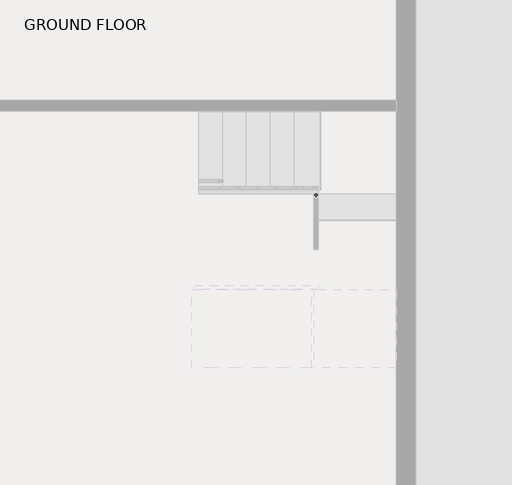
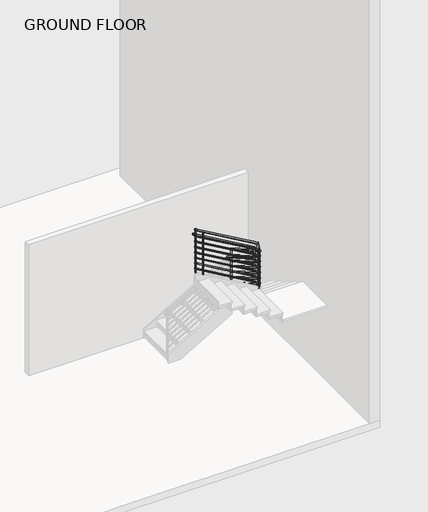
# One storey, part 2 of 3: 1 railing.
"""IFC4 building model written with IfcOpenShell, lengths in millimetres."""

from ifc_helpers import new_model, si_unit, frame, origin, place, context, project, spatial, circle_curve, ellipse_curve, element, save
from ifc_brep_helpers import plane_surface, cylinder_surface, advanced_brep

model = new_model("IFC4")

# Units and contexts
model_context = context("Model", 3, world=origin())
ifc_project = project(units=[si_unit("LENGTHUNIT", "METRE", prefix="MILLI")], contexts=[model_context])

# Site, building, storey
site = spatial("IfcSite", under=ifc_project)
building = spatial("IfcBuilding", under=site)
storey = spatial("IfcBuildingStorey", under=building, Name="GROUND FLOOR", Elevation=304.8)

# Railing
placement = place(None, origin())
element("IfcRailing", 1, ObjectType="Guardrail - Pipe", at=placement, inside=storey, context=model_context, shape_type="AdvancedBrep", body=[
    advanced_brep(
    [(2574.6930349, 4115.4555142, 2326.7540875), (2612.7930349, 4115.4555142, 2326.7540875), (2574.6930349, 3099.4555142, 2913.5348362), (2612.7930349, 3099.4555142, 2913.5348362)],
    [
        (0, 1, ellipse_curve(frame((2593.7430349, 4115.4555142, 2326.7540875), z_axis=(0.0, 1.0, 0.0), x_axis=(0.0, 0.0, -1.0)), 21.9988537, 19.05)),
        (1, 0, ellipse_curve(frame((2593.7430349, 4115.4555142, 2326.7540875), z_axis=(0.0, 1.0, 0.0), x_axis=(0.0, 0.0, -1.0)), 21.9988537, 19.05)),
        (2, 3, ellipse_curve(frame((2593.7430349, 3099.4555142, 2913.5348362), z_axis=(0.0, -0.49993835217939764, 0.8660609932447879), x_axis=(0.0, 0.866060993244788, 0.49993835217939775)), 21.9961413, 19.05)),
        (3, 2, ellipse_curve(frame((2593.7430349, 3099.4555142, 2913.5348362), z_axis=(0.0, -0.49993835217939764, 0.8660609932447879), x_axis=(0.0, 0.866060993244788, 0.49993835217939775)), 21.9961413, 19.05)),
        (0, 2),
        (3, 1),
    ],
    [
        plane_surface(frame((2593.7430349, 4115.4555142, 2348.7529412), z_axis=(0.0, 1.0, 0.0), x_axis=(0.0, 0.0, -1.0))),
        plane_surface(frame((2593.7430349, 3118.5055142, 2924.5315508), z_axis=(0.0, -0.49993835217939764, 0.8660609932447879), x_axis=(1.0, 0.0, 0.0))),
        cylinder_surface(frame((2593.7430349, 4105.9281656, 2332.2565134), z_axis=(0.0, 0.8659542116993035, -0.5001232880402972), x_axis=(1.0, 0.0, 0.0)), 19.05),
    ],
    [
        (0, [[1, 2]]),
        (1, [[3, 4]]),
        (2, [[-1, 5, -4, 6]]),
        (2, [[-2, -6, -3, -5]]),
    ],
),
    advanced_brep(
    [(2574.6930349, 3096.9019419, 2912.0607729), (2612.7930349, 3096.9019419, 2912.0607729), (2574.6930349, 3096.9019419, 3151.9199397), (2612.7930349, 3096.9019419, 3173.913369)],
    [
        (0, 1, ellipse_curve(frame((2593.7430349, 3096.9019419, 2912.0607729), z_axis=(0.0, 0.49993835217939764, -0.8660609932447879), x_axis=(0.0, -0.8660609932447879, -0.49993835217939775)), 21.9961413, 19.05)),
        (1, 0, ellipse_curve(frame((2593.7430349, 3096.9019419, 2912.0607729), z_axis=(0.0, 0.49993835217939764, -0.8660609932447879), x_axis=(0.0, -0.8660609932447879, -0.49993835217939775)), 21.9961413, 19.05)),
        (2, 3, ellipse_curve(frame((2593.7430349, 3096.9019419, 3162.9166543), z_axis=(-0.49993835217939775, 0.0, 0.8660609932447879), x_axis=(-0.8660609932447879, 0.0, -0.49993835217939764)), 21.9961413, 19.05)),
        (3, 2, ellipse_curve(frame((2593.7430349, 3096.9019419, 3162.9166543), z_axis=(-0.49993835217939775, 0.0, 0.8660609932447879), x_axis=(-0.8660609932447879, 0.0, -0.49993835217939764)), 21.9961413, 19.05)),
        (0, 2),
        (3, 1),
    ],
    [
        plane_surface(frame((2593.7430349, 3099.4555142, 2913.5348362), z_axis=(0.0, 0.49993835217939764, -0.8660609932447879), x_axis=(1.0, 0.0, 0.0))),
        plane_surface(frame((2593.7430349, 3099.4555142, 3162.9166543), z_axis=(-0.49993835217939775, 0.0, 0.8660609932447879), x_axis=(0.8660609932447879, 0.0, 0.49993835217939775))),
        cylinder_surface(frame((2593.7430349, 3096.9019419, 2913.5348362), z_axis=(0.0, 0.0, -1.0), x_axis=(1.0, 0.0, 0.0)), 19.05),
    ],
    [
        (0, [[1, 2]]),
        (1, [[3, 4]]),
        (2, [[-1, 5, -4, 6]]),
        (2, [[-2, -6, -3, -5]]),
    ],
),
    advanced_brep(
    [(2593.7430349, 3118.5055142, 3162.9166543), (2593.7430349, 3080.4055142, 3162.9166543), (1247.5430349, 3118.5055142, 3940.4011463), (1247.5430349, 3080.4055142, 3940.4011463)],
    [
        (0, 1, ellipse_curve(frame((2593.7430349, 3099.4555142, 3162.9166543), z_axis=(0.49993835217939775, 0.0, -0.8660609932447879), x_axis=(0.866060993244788, 0.0, 0.49993835217939786)), 21.9961413, 19.05)),
        (1, 0, ellipse_curve(frame((2593.7430349, 3099.4555142, 3162.9166543), z_axis=(0.49993835217939775, 0.0, -0.8660609932447879), x_axis=(0.866060993244788, 0.0, 0.49993835217939786)), 21.9961413, 19.05)),
        (2, 3, ellipse_curve(frame((1247.5430349, 3099.4555142, 3940.4011463), z_axis=(-1.0, 0.0, 0.0), x_axis=(0.0, 0.0, -1.0)), 21.9988537, 19.05)),
        (3, 2, ellipse_curve(frame((1247.5430349, 3099.4555142, 3940.4011463), z_axis=(-1.0, 0.0, 0.0), x_axis=(0.0, 0.0, -1.0)), 21.9988537, 19.05)),
        (0, 2),
        (3, 1),
    ],
    [
        plane_surface(frame((2612.7930349, 3099.4555142, 3173.913369), z_axis=(0.49993835217939775, 0.0, -0.8660609932447879), x_axis=(0.8660609932447879, 0.0, 0.49993835217939775))),
        plane_surface(frame((1247.5430349, 3099.4555142, 3962.4), z_axis=(-1.0, 0.0, 0.0), x_axis=(0.0, -1.0, 0.0))),
        cylinder_surface(frame((2603.2656863, 3099.4555142, 3157.4169413), z_axis=(0.8659542116993035, 0.0, -0.5001232880402972), x_axis=(0.0, -1.0, 0.0)), 19.05),
    ],
    [
        (0, [[1, 2]]),
        (1, [[3, 4]]),
        (2, [[-1, 5, -4, 6]]),
        (2, [[-2, -6, -3, -5]]),
    ],
),
    advanced_brep(
    [(2650.8930349, 4115.4555142, 2479.1540875), (2688.9930349, 4115.4555142, 2479.1540875), (2650.8930349, 3005.9999107, 3119.9091954), (2688.9930349, 3002.5661656, 3121.8923209)],
    [
        (0, 1, ellipse_curve(frame((2669.9430349, 4115.4555142, 2479.1540875), z_axis=(0.0, 1.0, 0.0), x_axis=(0.0, 0.0, -1.0)), 21.9988537, 19.05)),
        (1, 0, ellipse_curve(frame((2669.9430349, 4115.4555142, 2479.1540875), z_axis=(0.0, 1.0, 0.0), x_axis=(0.0, 0.0, -1.0)), 21.9988537, 19.05)),
        (2, 3, ellipse_curve(frame((2669.9430349, 3004.2830381, 3120.9007582), z_axis=(-0.0899527216771524, -0.5009550689581057, 0.8607859935826399), x_axis=(-0.15457437494221507, 0.8608390631720397, 0.4848328267849738)), 22.0408745, 19.05)),
        (3, 2, ellipse_curve(frame((2669.9430349, 3004.2830381, 3120.9007582), z_axis=(-0.0899527216771524, -0.5009550689581057, 0.8607859935826399), x_axis=(-0.15457437494221507, 0.8608390631720397, 0.4848328267849738)), 22.0408745, 19.05)),
        (0, 2),
        (3, 1),
    ],
    [
        plane_surface(frame((2669.9430349, 4115.4555142, 2501.1529412), z_axis=(0.0, 1.0, 0.0), x_axis=(0.0, 0.0, -1.0))),
        plane_surface(frame((2669.9430349, 3023.2555142, 3131.942246), z_axis=(-0.0899527216771524, -0.5009550689581057, 0.8607859935826399), x_axis=(0.995946036621901, -0.04524569628650927, 0.07774521917569083))),
        cylinder_surface(frame((2669.9430349, 4105.9281656, 2484.6565134), z_axis=(0.0, 0.8659542116993035, -0.5001232880402972), x_axis=(1.0, 0.0, 0.0)), 19.05),
    ],
    [
        (0, [[1, 2]]),
        (1, [[3, 4]]),
        (2, [[-1, 5, -4, 6]]),
        (2, [[-2, -6, -3, -5]]),
    ],
),
    advanced_brep(
    [(1247.5430349, 3042.3055142, 4092.8011463), (1247.5430349, 3004.2055142, 4092.8011463), (2649.2536863, 3042.3055142, 3155.5363184), (2652.6874314, 3004.2055142, 3133.7219377), (2627.1390822, 3042.3055142, 3296.0290977), (2627.1390822, 3004.2055142, 3296.0290977)],
    [
        (0, 1, ellipse_curve(frame((1247.5430349, 3023.2555142, 4092.8011463), z_axis=(-1.0, 0.0, 0.0), x_axis=(0.0, 0.0, -1.0)), 21.9988537, 19.05)),
        (1, 0, ellipse_curve(frame((1247.5430349, 3023.2555142, 4092.8011463), z_axis=(-1.0, 0.0, 0.0), x_axis=(0.0, 0.0, -1.0)), 21.9988537, 19.05)),
        (2, 3, ellipse_curve(frame((2650.9705589, 3023.2555142, 3144.6291281), z_axis=(0.0899527216771524, 0.5009550689581057, -0.8607859935826399), x_axis=(0.15457437494221501, -0.8608390631720398, -0.48483282678497347)), 22.0408745, 19.05)),
        (3, 2, ellipse_curve(frame((2650.9705589, 3023.2555142, 3144.6291281), z_axis=(0.0899527216771524, 0.5009550689581057, -0.8607859935826399), x_axis=(0.15457437494221501, -0.8608390631720398, -0.48483282678497347)), 22.0408745, 19.05)),
        (2, 4),
        (4, 5, ellipse_curve(frame((2627.1390822, 3023.2555142, 3296.0290977), z_axis=(0.5659546818459369, 0.0, -0.8244363517559525), x_axis=(-0.824436351755953, 0.0, -0.5659546818459362)), 21.110123, 19.05)),
        (5, 3),
        (5, 4, ellipse_curve(frame((2627.1390822, 3023.2555142, 3296.0290977), z_axis=(0.5659546818459369, 0.0, -0.8244363517559525), x_axis=(-0.824436351755953, 0.0, -0.5659546818459362)), 21.110123, 19.05)),
        (4, 0),
        (1, 5),
    ],
    [
        plane_surface(frame((1247.5430349, 3023.2555142, 4114.8), z_axis=(-1.0, 0.0, 0.0), x_axis=(0.0, -1.0, 0.0))),
        plane_surface(frame((2669.9430349, 3023.2555142, 3146.6117647), z_axis=(0.0899527216771524, 0.5009550689581057, -0.8607859935826399), x_axis=(0.995946036621901, -0.04524569628650927, 0.07774521917569083))),
        cylinder_surface(frame((2651.1247398, 3023.2555142, 3143.6496257), z_axis=(0.1554928635658915, 0.0, -0.9878370155952242), x_axis=(0.0, -1.0, 0.0)), 19.05),
        cylinder_surface(frame((2635.0156863, 3023.2555142, 3291.4800429), z_axis=(0.8659542116993035, 0.0, -0.500123288040297), x_axis=(0.0, -1.0, 0.0)), 19.05),
    ],
    [
        (0, [[1, 2]]),
        (1, [[3, 4]]),
        (2, [[-3, 5, 6, 7]]),
        (2, [[-4, -7, 8, -5]]),
        (3, [[-6, 9, -2, 10]]),
        (3, [[-8, -10, -1, -9]]),
    ],
),
    advanced_brep(
    [(2657.2430349, 4115.4555142, 2334.0870387), (2682.6430349, 4115.4555142, 2334.0870387), (2657.2430349, 3035.9555142, 2957.5415842), (2682.6430349, 3035.9555142, 2957.5415842)],
    [
        (0, 1, ellipse_curve(frame((2669.9430349, 4115.4555142, 2334.0870387), z_axis=(0.0, 1.0, 0.0), x_axis=(0.0, 0.0, -1.0)), 14.6659025, 12.7)),
        (1, 0, ellipse_curve(frame((2669.9430349, 4115.4555142, 2334.0870387), z_axis=(0.0, 1.0, 0.0), x_axis=(0.0, 0.0, -1.0)), 14.6659025, 12.7)),
        (2, 3, ellipse_curve(frame((2669.9430349, 3035.9555142, 2957.5415842), z_axis=(0.0, -1.0, 0.0), x_axis=(0.0, 0.0, -1.0)), 14.6659025, 12.7)),
        (3, 2, ellipse_curve(frame((2669.9430349, 3035.9555142, 2957.5415842), z_axis=(0.0, -1.0, 0.0), x_axis=(0.0, 0.0, -1.0)), 14.6659025, 12.7)),
        (0, 2),
        (3, 1),
    ],
    [
        plane_surface(frame((2669.9430349, 4115.4555142, 2348.7529412), z_axis=(0.0, 1.0, 0.0), x_axis=(0.0, 0.0, -1.0))),
        plane_surface(frame((2669.9430349, 3035.9555142, 2972.2074866), z_axis=(0.0, -1.0, 0.0), x_axis=(0.0, 0.0, -1.0))),
        cylinder_surface(frame((2669.9430349, 4109.1039485, 2337.7553227), z_axis=(0.0, 0.8659542116993035, -0.5001232880402972), x_axis=(1.0, 0.0, 0.0)), 12.7),
    ],
    [
        (0, [[1, 2]]),
        (1, [[3, 4]]),
        (2, [[-1, 5, -4, 6]]),
        (2, [[-2, -6, -3, -5]]),
    ],
),
    advanced_brep(
    [(2682.6430349, 3035.9555142, 2981.5117647), (2682.6430349, 3010.5555142, 2981.5117647), (2659.0857372, 3035.9555142, 2981.5117647), (2659.0857372, 3010.5555142, 2981.5117647), (2644.5430349, 3035.9555142, 3073.9006965), (2644.5430349, 3010.5555142, 3073.9006965)],
    [
        (0, 1, circle_curve(frame((2682.6430349, 3023.2555142, 2981.5117647), z_axis=(1.0, 0.0, 0.0), x_axis=(0.0, -1.0, 0.0)), 12.7)),
        (1, 0, circle_curve(frame((2682.6430349, 3023.2555142, 2981.5117647), z_axis=(1.0, 0.0, 0.0), x_axis=(0.0, -1.0, 0.0)), 12.7)),
        (0, 2),
        (2, 3, ellipse_curve(frame((2659.0857372, 3023.2555142, 2981.5117647), z_axis=(0.7600963305943172, 0.0, -0.6498104094403646), x_axis=(0.6498104094403648, 0.0, 0.7600963305943174)), 16.7084085, 12.7)),
        (3, 1),
        (3, 2, ellipse_curve(frame((2659.0857372, 3023.2555142, 2981.5117647), z_axis=(0.7600963305943172, 0.0, -0.6498104094403646), x_axis=(0.6498104094403648, 0.0, 0.7600963305943174)), 16.7084085, 12.7)),
        (4, 5, ellipse_curve(frame((2644.5430349, 3023.2555142, 3073.9006965), z_axis=(-1.0, 0.0, 0.0), x_axis=(0.0, 0.0, -1.0)), 81.6757741, 12.7)),
        (5, 4, ellipse_curve(frame((2644.5430349, 3023.2555142, 3073.9006965), z_axis=(-1.0, 0.0, 0.0), x_axis=(0.0, 0.0, -1.0)), 81.6757741, 12.7)),
        (2, 4),
        (5, 3),
    ],
    [
        plane_surface(frame((2682.6430349, 3023.2555142, 2994.2117647), z_axis=(1.0, 0.0, 0.0), x_axis=(0.0, -1.0, 0.0))),
        cylinder_surface(frame((2682.6430349, 3023.2555142, 2981.5117647), z_axis=(1.0, 0.0, 0.0), x_axis=(0.0, -1.0, 0.0)), 12.7),
        plane_surface(frame((2644.5430349, 3023.2555142, 3155.5764706), z_axis=(-1.0, 0.0, 0.0), x_axis=(0.0, -1.0, 0.0))),
        cylinder_surface(frame((2657.3975048, 3023.2555142, 2992.2370053), z_axis=(0.15549286356589131, 0.0, -0.9878370155952242), x_axis=(0.0, -1.0, 0.0)), 12.7),
    ],
    [
        (0, [[1, 2]]),
        (1, [[-1, 3, 4, 5]]),
        (1, [[-2, -5, 6, -3]]),
        (2, [[7, 8]]),
        (3, [[-4, 9, -8, 10]]),
        (3, [[-6, -10, -7, -9]]),
    ],
),
    advanced_brep(
    [(2644.5430349, 3035.9555142, 3140.9105681), (2644.5430349, 3010.5555142, 3140.9105681), (1247.5430349, 3035.9555142, 3947.7340975), (1247.5430349, 3010.5555142, 3947.7340975)],
    [
        (0, 1, ellipse_curve(frame((2644.5430349, 3023.2555142, 3140.9105681), z_axis=(1.0, 0.0, 0.0), x_axis=(0.0, 0.0, -1.0)), 14.6659025, 12.7)),
        (1, 0, ellipse_curve(frame((2644.5430349, 3023.2555142, 3140.9105681), z_axis=(1.0, 0.0, 0.0), x_axis=(0.0, 0.0, -1.0)), 14.6659025, 12.7)),
        (2, 3, ellipse_curve(frame((1247.5430349, 3023.2555142, 3947.7340975), z_axis=(-1.0, 0.0, 0.0), x_axis=(0.0, 0.0, -1.0)), 14.6659025, 12.7)),
        (3, 2, ellipse_curve(frame((1247.5430349, 3023.2555142, 3947.7340975), z_axis=(-1.0, 0.0, 0.0), x_axis=(0.0, 0.0, -1.0)), 14.6659025, 12.7)),
        (0, 2),
        (3, 1),
    ],
    [
        plane_surface(frame((2644.5430349, 3023.2555142, 3155.5764706), z_axis=(1.0, 0.0, 0.0), x_axis=(0.0, -1.0, 0.0))),
        plane_surface(frame((1247.5430349, 3023.2555142, 3962.4), z_axis=(-1.0, 0.0, 0.0), x_axis=(0.0, -1.0, 0.0))),
        cylinder_surface(frame((2638.1914692, 3023.2555142, 3144.5788521), z_axis=(0.8659542116993035, 0.0, -0.5001232880402972), x_axis=(0.0, -1.0, 0.0)), 12.7),
    ],
    [
        (0, [[1, 2]]),
        (1, [[3, 4]]),
        (2, [[-1, 5, -4, 6]]),
        (2, [[-2, -6, -3, -5]]),
    ],
),
    advanced_brep(
    [(2657.2430349, 4115.4555142, 2207.0870387), (2682.6430349, 4115.4555142, 2207.0870387), (2657.2430349, 3035.9555142, 2830.5415842), (2682.6430349, 3035.9555142, 2830.5415842)],
    [
        (0, 1, ellipse_curve(frame((2669.9430349, 4115.4555142, 2207.0870387), z_axis=(0.0, 1.0, 0.0), x_axis=(0.0, 0.0, -1.0)), 14.6659025, 12.7)),
        (1, 0, ellipse_curve(frame((2669.9430349, 4115.4555142, 2207.0870387), z_axis=(0.0, 1.0, 0.0), x_axis=(0.0, 0.0, -1.0)), 14.6659025, 12.7)),
        (2, 3, ellipse_curve(frame((2669.9430349, 3035.9555142, 2830.5415842), z_axis=(0.0, -1.0, 0.0), x_axis=(0.0, 0.0, -1.0)), 14.6659025, 12.7)),
        (3, 2, ellipse_curve(frame((2669.9430349, 3035.9555142, 2830.5415842), z_axis=(0.0, -1.0, 0.0), x_axis=(0.0, 0.0, -1.0)), 14.6659025, 12.7)),
        (0, 2),
        (3, 1),
    ],
    [
        plane_surface(frame((2669.9430349, 4115.4555142, 2221.7529412), z_axis=(0.0, 1.0, 0.0), x_axis=(0.0, 0.0, -1.0))),
        plane_surface(frame((2669.9430349, 3035.9555142, 2845.2074866), z_axis=(0.0, -1.0, 0.0), x_axis=(0.0, 0.0, -1.0))),
        cylinder_surface(frame((2669.9430349, 4109.1039485, 2210.7553227), z_axis=(0.0, 0.8659542116993035, -0.5001232880402972), x_axis=(1.0, 0.0, 0.0)), 12.7),
    ],
    [
        (0, [[1, 2]]),
        (1, [[3, 4]]),
        (2, [[-1, 5, -4, 6]]),
        (2, [[-2, -6, -3, -5]]),
    ],
),
    advanced_brep(
    [(2682.6430349, 3035.9555142, 2854.5117647), (2682.6430349, 3010.5555142, 2854.5117647), (2659.0857372, 3035.9555142, 2854.5117647), (2659.0857372, 3010.5555142, 2854.5117647), (2644.5430349, 3035.9555142, 2946.9006965), (2644.5430349, 3010.5555142, 2946.9006965)],
    [
        (0, 1, circle_curve(frame((2682.6430349, 3023.2555142, 2854.5117647), z_axis=(1.0, 0.0, 0.0), x_axis=(0.0, -1.0, 0.0)), 12.7)),
        (1, 0, circle_curve(frame((2682.6430349, 3023.2555142, 2854.5117647), z_axis=(1.0, 0.0, 0.0), x_axis=(0.0, -1.0, 0.0)), 12.7)),
        (0, 2),
        (2, 3, ellipse_curve(frame((2659.0857372, 3023.2555142, 2854.5117647), z_axis=(0.7600963305943172, 0.0, -0.6498104094403646), x_axis=(0.6498104094403648, 0.0, 0.7600963305943174)), 16.7084085, 12.7)),
        (3, 1),
        (3, 2, ellipse_curve(frame((2659.0857372, 3023.2555142, 2854.5117647), z_axis=(0.7600963305943172, 0.0, -0.6498104094403646), x_axis=(0.6498104094403648, 0.0, 0.7600963305943174)), 16.7084085, 12.7)),
        (4, 5, ellipse_curve(frame((2644.5430349, 3023.2555142, 2946.9006965), z_axis=(-1.0, 0.0, 0.0), x_axis=(0.0, 0.0, -1.0)), 81.6757741, 12.7)),
        (5, 4, ellipse_curve(frame((2644.5430349, 3023.2555142, 2946.9006965), z_axis=(-1.0, 0.0, 0.0), x_axis=(0.0, 0.0, -1.0)), 81.6757741, 12.7)),
        (2, 4),
        (5, 3),
    ],
    [
        plane_surface(frame((2682.6430349, 3023.2555142, 2867.2117647), z_axis=(1.0, 0.0, 0.0), x_axis=(0.0, -1.0, 0.0))),
        cylinder_surface(frame((2682.6430349, 3023.2555142, 2854.5117647), z_axis=(1.0, 0.0, 0.0), x_axis=(0.0, -1.0, 0.0)), 12.7),
        plane_surface(frame((2644.5430349, 3023.2555142, 3028.5764706), z_axis=(-1.0, 0.0, 0.0), x_axis=(0.0, -1.0, 0.0))),
        cylinder_surface(frame((2657.3975048, 3023.2555142, 2865.2370053), z_axis=(0.15549286356589131, 0.0, -0.9878370155952242), x_axis=(0.0, -1.0, 0.0)), 12.7),
    ],
    [
        (0, [[1, 2]]),
        (1, [[-1, 3, 4, 5]]),
        (1, [[-2, -5, 6, -3]]),
        (2, [[7, 8]]),
        (3, [[-4, 9, -8, 10]]),
        (3, [[-6, -10, -7, -9]]),
    ],
),
    advanced_brep(
    [(2644.5430349, 3035.9555142, 3013.9105681), (2644.5430349, 3010.5555142, 3013.9105681), (1247.5430349, 3035.9555142, 3820.7340975), (1247.5430349, 3010.5555142, 3820.7340975)],
    [
        (0, 1, ellipse_curve(frame((2644.5430349, 3023.2555142, 3013.9105681), z_axis=(1.0, 0.0, 0.0), x_axis=(0.0, 0.0, -1.0)), 14.6659025, 12.7)),
        (1, 0, ellipse_curve(frame((2644.5430349, 3023.2555142, 3013.9105681), z_axis=(1.0, 0.0, 0.0), x_axis=(0.0, 0.0, -1.0)), 14.6659025, 12.7)),
        (2, 3, ellipse_curve(frame((1247.5430349, 3023.2555142, 3820.7340975), z_axis=(-1.0, 0.0, 0.0), x_axis=(0.0, 0.0, -1.0)), 14.6659025, 12.7)),
        (3, 2, ellipse_curve(frame((1247.5430349, 3023.2555142, 3820.7340975), z_axis=(-1.0, 0.0, 0.0), x_axis=(0.0, 0.0, -1.0)), 14.6659025, 12.7)),
        (0, 2),
        (3, 1),
    ],
    [
        plane_surface(frame((2644.5430349, 3023.2555142, 3028.5764706), z_axis=(1.0, 0.0, 0.0), x_axis=(0.0, -1.0, 0.0))),
        plane_surface(frame((1247.5430349, 3023.2555142, 3835.4), z_axis=(-1.0, 0.0, 0.0), x_axis=(0.0, -1.0, 0.0))),
        cylinder_surface(frame((2638.1914692, 3023.2555142, 3017.5788521), z_axis=(0.8659542116993035, 0.0, -0.5001232880402972), x_axis=(0.0, -1.0, 0.0)), 12.7),
    ],
    [
        (0, [[1, 2]]),
        (1, [[3, 4]]),
        (2, [[-1, 5, -4, 6]]),
        (2, [[-2, -6, -3, -5]]),
    ],
),
    advanced_brep(
    [(2657.2430349, 4115.4555142, 2080.0870387), (2682.6430349, 4115.4555142, 2080.0870387), (2657.2430349, 3035.9555142, 2703.5415842), (2682.6430349, 3035.9555142, 2703.5415842)],
    [
        (0, 1, ellipse_curve(frame((2669.9430349, 4115.4555142, 2080.0870387), z_axis=(0.0, 1.0, 0.0), x_axis=(0.0, 0.0, -1.0)), 14.6659025, 12.7)),
        (1, 0, ellipse_curve(frame((2669.9430349, 4115.4555142, 2080.0870387), z_axis=(0.0, 1.0, 0.0), x_axis=(0.0, 0.0, -1.0)), 14.6659025, 12.7)),
        (2, 3, ellipse_curve(frame((2669.9430349, 3035.9555142, 2703.5415842), z_axis=(0.0, -1.0, 0.0), x_axis=(0.0, 0.0, -1.0)), 14.6659025, 12.7)),
        (3, 2, ellipse_curve(frame((2669.9430349, 3035.9555142, 2703.5415842), z_axis=(0.0, -1.0, 0.0), x_axis=(0.0, 0.0, -1.0)), 14.6659025, 12.7)),
        (0, 2),
        (3, 1),
    ],
    [
        plane_surface(frame((2669.9430349, 4115.4555142, 2094.7529412), z_axis=(0.0, 1.0, 0.0), x_axis=(0.0, 0.0, -1.0))),
        plane_surface(frame((2669.9430349, 3035.9555142, 2718.2074866), z_axis=(0.0, -1.0, 0.0), x_axis=(0.0, 0.0, -1.0))),
        cylinder_surface(frame((2669.9430349, 4109.1039485, 2083.7553227), z_axis=(0.0, 0.8659542116993035, -0.5001232880402972), x_axis=(1.0, 0.0, 0.0)), 12.7),
    ],
    [
        (0, [[1, 2]]),
        (1, [[3, 4]]),
        (2, [[-1, 5, -4, 6]]),
        (2, [[-2, -6, -3, -5]]),
    ],
),
    advanced_brep(
    [(2682.6430349, 3035.9555142, 2727.5117647), (2682.6430349, 3010.5555142, 2727.5117647), (2659.0857372, 3035.9555142, 2727.5117647), (2659.0857372, 3010.5555142, 2727.5117647), (2644.5430349, 3035.9555142, 2819.9006965), (2644.5430349, 3010.5555142, 2819.9006965)],
    [
        (0, 1, circle_curve(frame((2682.6430349, 3023.2555142, 2727.5117647), z_axis=(1.0, 0.0, 0.0), x_axis=(0.0, -1.0, 0.0)), 12.7)),
        (1, 0, circle_curve(frame((2682.6430349, 3023.2555142, 2727.5117647), z_axis=(1.0, 0.0, 0.0), x_axis=(0.0, -1.0, 0.0)), 12.7)),
        (0, 2),
        (2, 3, ellipse_curve(frame((2659.0857372, 3023.2555142, 2727.5117647), z_axis=(0.7600963305943172, 0.0, -0.6498104094403646), x_axis=(0.6498104094403648, 0.0, 0.7600963305943174)), 16.7084085, 12.7)),
        (3, 1),
        (3, 2, ellipse_curve(frame((2659.0857372, 3023.2555142, 2727.5117647), z_axis=(0.7600963305943172, 0.0, -0.6498104094403646), x_axis=(0.6498104094403648, 0.0, 0.7600963305943174)), 16.7084085, 12.7)),
        (4, 5, ellipse_curve(frame((2644.5430349, 3023.2555142, 2819.9006965), z_axis=(-1.0, 0.0, 0.0), x_axis=(0.0, 0.0, -1.0)), 81.6757741, 12.7)),
        (5, 4, ellipse_curve(frame((2644.5430349, 3023.2555142, 2819.9006965), z_axis=(-1.0, 0.0, 0.0), x_axis=(0.0, 0.0, -1.0)), 81.6757741, 12.7)),
        (2, 4),
        (5, 3),
    ],
    [
        plane_surface(frame((2682.6430349, 3023.2555142, 2740.2117647), z_axis=(1.0, 0.0, 0.0), x_axis=(0.0, -1.0, 0.0))),
        cylinder_surface(frame((2682.6430349, 3023.2555142, 2727.5117647), z_axis=(1.0, 0.0, 0.0), x_axis=(0.0, -1.0, 0.0)), 12.7),
        plane_surface(frame((2644.5430349, 3023.2555142, 2901.5764706), z_axis=(-1.0, 0.0, 0.0), x_axis=(0.0, -1.0, 0.0))),
        cylinder_surface(frame((2657.3975048, 3023.2555142, 2738.2370053), z_axis=(0.15549286356589131, 0.0, -0.9878370155952242), x_axis=(0.0, -1.0, 0.0)), 12.7),
    ],
    [
        (0, [[1, 2]]),
        (1, [[-1, 3, 4, 5]]),
        (1, [[-2, -5, 6, -3]]),
        (2, [[7, 8]]),
        (3, [[-4, 9, -8, 10]]),
        (3, [[-6, -10, -7, -9]]),
    ],
),
    advanced_brep(
    [(2644.5430349, 3035.9555142, 2886.9105681), (2644.5430349, 3010.5555142, 2886.9105681), (1247.5430349, 3035.9555142, 3693.7340975), (1247.5430349, 3010.5555142, 3693.7340975)],
    [
        (0, 1, ellipse_curve(frame((2644.5430349, 3023.2555142, 2886.9105681), z_axis=(1.0, 0.0, 0.0), x_axis=(0.0, 0.0, -1.0)), 14.6659025, 12.7)),
        (1, 0, ellipse_curve(frame((2644.5430349, 3023.2555142, 2886.9105681), z_axis=(1.0, 0.0, 0.0), x_axis=(0.0, 0.0, -1.0)), 14.6659025, 12.7)),
        (2, 3, ellipse_curve(frame((1247.5430349, 3023.2555142, 3693.7340975), z_axis=(-1.0, 0.0, 0.0), x_axis=(0.0, 0.0, -1.0)), 14.6659025, 12.7)),
        (3, 2, ellipse_curve(frame((1247.5430349, 3023.2555142, 3693.7340975), z_axis=(-1.0, 0.0, 0.0), x_axis=(0.0, 0.0, -1.0)), 14.6659025, 12.7)),
        (0, 2),
        (3, 1),
    ],
    [
        plane_surface(frame((2644.5430349, 3023.2555142, 2901.5764706), z_axis=(1.0, 0.0, 0.0), x_axis=(0.0, -1.0, 0.0))),
        plane_surface(frame((1247.5430349, 3023.2555142, 3708.4), z_axis=(-1.0, 0.0, 0.0), x_axis=(0.0, -1.0, 0.0))),
        cylinder_surface(frame((2638.1914692, 3023.2555142, 2890.5788521), z_axis=(0.8659542116993035, 0.0, -0.5001232880402972), x_axis=(0.0, -1.0, 0.0)), 12.7),
    ],
    [
        (0, [[1, 2]]),
        (1, [[3, 4]]),
        (2, [[-1, 5, -4, 6]]),
        (2, [[-2, -6, -3, -5]]),
    ],
),
    advanced_brep(
    [(2657.2430349, 4115.4555142, 1953.0870387), (2682.6430349, 4115.4555142, 1953.0870387), (2657.2430349, 3035.9555142, 2576.5415842), (2682.6430349, 3035.9555142, 2576.5415842)],
    [
        (0, 1, ellipse_curve(frame((2669.9430349, 4115.4555142, 1953.0870387), z_axis=(0.0, 1.0, 0.0), x_axis=(0.0, 0.0, -1.0)), 14.6659025, 12.7)),
        (1, 0, ellipse_curve(frame((2669.9430349, 4115.4555142, 1953.0870387), z_axis=(0.0, 1.0, 0.0), x_axis=(0.0, 0.0, -1.0)), 14.6659025, 12.7)),
        (2, 3, ellipse_curve(frame((2669.9430349, 3035.9555142, 2576.5415842), z_axis=(0.0, -1.0, 0.0), x_axis=(0.0, 0.0, -1.0)), 14.6659025, 12.7)),
        (3, 2, ellipse_curve(frame((2669.9430349, 3035.9555142, 2576.5415842), z_axis=(0.0, -1.0, 0.0), x_axis=(0.0, 0.0, -1.0)), 14.6659025, 12.7)),
        (0, 2),
        (3, 1),
    ],
    [
        plane_surface(frame((2669.9430349, 4115.4555142, 1967.7529412), z_axis=(0.0, 1.0, 0.0), x_axis=(0.0, 0.0, -1.0))),
        plane_surface(frame((2669.9430349, 3035.9555142, 2591.2074866), z_axis=(0.0, -1.0, 0.0), x_axis=(0.0, 0.0, -1.0))),
        cylinder_surface(frame((2669.9430349, 4109.1039485, 1956.7553227), z_axis=(0.0, 0.8659542116993035, -0.5001232880402972), x_axis=(1.0, 0.0, 0.0)), 12.7),
    ],
    [
        (0, [[1, 2]]),
        (1, [[3, 4]]),
        (2, [[-1, 5, -4, 6]]),
        (2, [[-2, -6, -3, -5]]),
    ],
),
    advanced_brep(
    [(2682.6430349, 3035.9555142, 2600.5117647), (2682.6430349, 3010.5555142, 2600.5117647), (2659.0857372, 3035.9555142, 2600.5117647), (2659.0857372, 3010.5555142, 2600.5117647), (2644.5430349, 3035.9555142, 2692.9006965), (2644.5430349, 3010.5555142, 2692.9006965)],
    [
        (0, 1, circle_curve(frame((2682.6430349, 3023.2555142, 2600.5117647), z_axis=(1.0, 0.0, 0.0), x_axis=(0.0, -1.0, 0.0)), 12.7)),
        (1, 0, circle_curve(frame((2682.6430349, 3023.2555142, 2600.5117647), z_axis=(1.0, 0.0, 0.0), x_axis=(0.0, -1.0, 0.0)), 12.7)),
        (0, 2),
        (2, 3, ellipse_curve(frame((2659.0857372, 3023.2555142, 2600.5117647), z_axis=(0.7600963305943172, 0.0, -0.6498104094403646), x_axis=(0.6498104094403648, 0.0, 0.7600963305943174)), 16.7084085, 12.7)),
        (3, 1),
        (3, 2, ellipse_curve(frame((2659.0857372, 3023.2555142, 2600.5117647), z_axis=(0.7600963305943172, 0.0, -0.6498104094403646), x_axis=(0.6498104094403648, 0.0, 0.7600963305943174)), 16.7084085, 12.7)),
        (4, 5, ellipse_curve(frame((2644.5430349, 3023.2555142, 2692.9006965), z_axis=(-1.0, 0.0, 0.0), x_axis=(0.0, 0.0, -1.0)), 81.6757741, 12.7)),
        (5, 4, ellipse_curve(frame((2644.5430349, 3023.2555142, 2692.9006965), z_axis=(-1.0, 0.0, 0.0), x_axis=(0.0, 0.0, -1.0)), 81.6757741, 12.7)),
        (2, 4),
        (5, 3),
    ],
    [
        plane_surface(frame((2682.6430349, 3023.2555142, 2613.2117647), z_axis=(1.0, 0.0, 0.0), x_axis=(0.0, -1.0, 0.0))),
        cylinder_surface(frame((2682.6430349, 3023.2555142, 2600.5117647), z_axis=(1.0, 0.0, 0.0), x_axis=(0.0, -1.0, 0.0)), 12.7),
        plane_surface(frame((2644.5430349, 3023.2555142, 2774.5764706), z_axis=(-1.0, 0.0, 0.0), x_axis=(0.0, -1.0, 0.0))),
        cylinder_surface(frame((2657.3975048, 3023.2555142, 2611.2370053), z_axis=(0.15549286356589131, 0.0, -0.9878370155952242), x_axis=(0.0, -1.0, 0.0)), 12.7),
    ],
    [
        (0, [[1, 2]]),
        (1, [[-1, 3, 4, 5]]),
        (1, [[-2, -5, 6, -3]]),
        (2, [[7, 8]]),
        (3, [[-4, 9, -8, 10]]),
        (3, [[-6, -10, -7, -9]]),
    ],
),
    advanced_brep(
    [(2644.5430349, 3035.9555142, 2759.9105681), (2644.5430349, 3010.5555142, 2759.9105681), (1247.5430349, 3035.9555142, 3566.7340975), (1247.5430349, 3010.5555142, 3566.7340975)],
    [
        (0, 1, ellipse_curve(frame((2644.5430349, 3023.2555142, 2759.9105681), z_axis=(1.0, 0.0, 0.0), x_axis=(0.0, 0.0, -1.0)), 14.6659025, 12.7)),
        (1, 0, ellipse_curve(frame((2644.5430349, 3023.2555142, 2759.9105681), z_axis=(1.0, 0.0, 0.0), x_axis=(0.0, 0.0, -1.0)), 14.6659025, 12.7)),
        (2, 3, ellipse_curve(frame((1247.5430349, 3023.2555142, 3566.7340975), z_axis=(-1.0, 0.0, 0.0), x_axis=(0.0, 0.0, -1.0)), 14.6659025, 12.7)),
        (3, 2, ellipse_curve(frame((1247.5430349, 3023.2555142, 3566.7340975), z_axis=(-1.0, 0.0, 0.0), x_axis=(0.0, 0.0, -1.0)), 14.6659025, 12.7)),
        (0, 2),
        (3, 1),
    ],
    [
        plane_surface(frame((2644.5430349, 3023.2555142, 2774.5764706), z_axis=(1.0, 0.0, 0.0), x_axis=(0.0, -1.0, 0.0))),
        plane_surface(frame((1247.5430349, 3023.2555142, 3581.4), z_axis=(-1.0, 0.0, 0.0), x_axis=(0.0, -1.0, 0.0))),
        cylinder_surface(frame((2638.1914692, 3023.2555142, 2763.5788521), z_axis=(0.8659542116993035, 0.0, -0.5001232880402972), x_axis=(0.0, -1.0, 0.0)), 12.7),
    ],
    [
        (0, [[1, 2]]),
        (1, [[3, 4]]),
        (2, [[-1, 5, -4, 6]]),
        (2, [[-2, -6, -3, -5]]),
    ],
),
    advanced_brep(
    [(2657.2430349, 4115.4555142, 1826.0870387), (2682.6430349, 4115.4555142, 1826.0870387), (2657.2430349, 3035.9555142, 2449.5415842), (2682.6430349, 3035.9555142, 2449.5415842)],
    [
        (0, 1, ellipse_curve(frame((2669.9430349, 4115.4555142, 1826.0870387), z_axis=(0.0, 1.0, 0.0), x_axis=(0.0, 0.0, -1.0)), 14.6659025, 12.7)),
        (1, 0, ellipse_curve(frame((2669.9430349, 4115.4555142, 1826.0870387), z_axis=(0.0, 1.0, 0.0), x_axis=(0.0, 0.0, -1.0)), 14.6659025, 12.7)),
        (2, 3, ellipse_curve(frame((2669.9430349, 3035.9555142, 2449.5415842), z_axis=(0.0, -1.0, 0.0), x_axis=(0.0, 0.0, -1.0)), 14.6659025, 12.7)),
        (3, 2, ellipse_curve(frame((2669.9430349, 3035.9555142, 2449.5415842), z_axis=(0.0, -1.0, 0.0), x_axis=(0.0, 0.0, -1.0)), 14.6659025, 12.7)),
        (0, 2),
        (3, 1),
    ],
    [
        plane_surface(frame((2669.9430349, 4115.4555142, 1840.7529412), z_axis=(0.0, 1.0, 0.0), x_axis=(0.0, 0.0, -1.0))),
        plane_surface(frame((2669.9430349, 3035.9555142, 2464.2074866), z_axis=(0.0, -1.0, 0.0), x_axis=(0.0, 0.0, -1.0))),
        cylinder_surface(frame((2669.9430349, 4109.1039485, 1829.7553227), z_axis=(0.0, 0.8659542116993035, -0.5001232880402972), x_axis=(1.0, 0.0, 0.0)), 12.7),
    ],
    [
        (0, [[1, 2]]),
        (1, [[3, 4]]),
        (2, [[-1, 5, -4, 6]]),
        (2, [[-2, -6, -3, -5]]),
    ],
),
    advanced_brep(
    [(2682.6430349, 3035.9555142, 2473.5117647), (2682.6430349, 3010.5555142, 2473.5117647), (2659.0857372, 3035.9555142, 2473.5117647), (2659.0857372, 3010.5555142, 2473.5117647), (2644.5430349, 3035.9555142, 2565.9006965), (2644.5430349, 3010.5555142, 2565.9006965)],
    [
        (0, 1, circle_curve(frame((2682.6430349, 3023.2555142, 2473.5117647), z_axis=(1.0, 0.0, 0.0), x_axis=(0.0, -1.0, 0.0)), 12.7)),
        (1, 0, circle_curve(frame((2682.6430349, 3023.2555142, 2473.5117647), z_axis=(1.0, 0.0, 0.0), x_axis=(0.0, -1.0, 0.0)), 12.7)),
        (0, 2),
        (2, 3, ellipse_curve(frame((2659.0857372, 3023.2555142, 2473.5117647), z_axis=(0.7600963305943172, 0.0, -0.6498104094403646), x_axis=(0.6498104094403648, 0.0, 0.7600963305943174)), 16.7084085, 12.7)),
        (3, 1),
        (3, 2, ellipse_curve(frame((2659.0857372, 3023.2555142, 2473.5117647), z_axis=(0.7600963305943172, 0.0, -0.6498104094403646), x_axis=(0.6498104094403648, 0.0, 0.7600963305943174)), 16.7084085, 12.7)),
        (4, 5, ellipse_curve(frame((2644.5430349, 3023.2555142, 2565.9006965), z_axis=(-1.0, 0.0, 0.0), x_axis=(0.0, 0.0, -1.0)), 81.6757741, 12.7)),
        (5, 4, ellipse_curve(frame((2644.5430349, 3023.2555142, 2565.9006965), z_axis=(-1.0, 0.0, 0.0), x_axis=(0.0, 0.0, -1.0)), 81.6757741, 12.7)),
        (2, 4),
        (5, 3),
    ],
    [
        plane_surface(frame((2682.6430349, 3023.2555142, 2486.2117647), z_axis=(1.0, 0.0, 0.0), x_axis=(0.0, -1.0, 0.0))),
        cylinder_surface(frame((2682.6430349, 3023.2555142, 2473.5117647), z_axis=(1.0, 0.0, 0.0), x_axis=(0.0, -1.0, 0.0)), 12.7),
        plane_surface(frame((2644.5430349, 3023.2555142, 2647.5764706), z_axis=(-1.0, 0.0, 0.0), x_axis=(0.0, -1.0, 0.0))),
        cylinder_surface(frame((2657.3975048, 3023.2555142, 2484.2370053), z_axis=(0.15549286356589131, 0.0, -0.9878370155952242), x_axis=(0.0, -1.0, 0.0)), 12.7),
    ],
    [
        (0, [[1, 2]]),
        (1, [[-1, 3, 4, 5]]),
        (1, [[-2, -5, 6, -3]]),
        (2, [[7, 8]]),
        (3, [[-4, 9, -8, 10]]),
        (3, [[-6, -10, -7, -9]]),
    ],
),
    advanced_brep(
    [(2644.5430349, 3035.9555142, 2632.9105681), (2644.5430349, 3010.5555142, 2632.9105681), (1247.5430349, 3035.9555142, 3439.7340975), (1247.5430349, 3010.5555142, 3439.7340975)],
    [
        (0, 1, ellipse_curve(frame((2644.5430349, 3023.2555142, 2632.9105681), z_axis=(1.0, 0.0, 0.0), x_axis=(0.0, 0.0, -1.0)), 14.6659025, 12.7)),
        (1, 0, ellipse_curve(frame((2644.5430349, 3023.2555142, 2632.9105681), z_axis=(1.0, 0.0, 0.0), x_axis=(0.0, 0.0, -1.0)), 14.6659025, 12.7)),
        (2, 3, ellipse_curve(frame((1247.5430349, 3023.2555142, 3439.7340975), z_axis=(-1.0, 0.0, 0.0), x_axis=(0.0, 0.0, -1.0)), 14.6659025, 12.7)),
        (3, 2, ellipse_curve(frame((1247.5430349, 3023.2555142, 3439.7340975), z_axis=(-1.0, 0.0, 0.0), x_axis=(0.0, 0.0, -1.0)), 14.6659025, 12.7)),
        (0, 2),
        (3, 1),
    ],
    [
        plane_surface(frame((2644.5430349, 3023.2555142, 2647.5764706), z_axis=(1.0, 0.0, 0.0), x_axis=(0.0, -1.0, 0.0))),
        plane_surface(frame((1247.5430349, 3023.2555142, 3454.4), z_axis=(-1.0, 0.0, 0.0), x_axis=(0.0, -1.0, 0.0))),
        cylinder_surface(frame((2638.1914692, 3023.2555142, 2636.5788521), z_axis=(0.8659542116993035, 0.0, -0.5001232880402972), x_axis=(0.0, -1.0, 0.0)), 12.7),
    ],
    [
        (0, [[1, 2]]),
        (1, [[3, 4]]),
        (2, [[-1, 5, -4, 6]]),
        (2, [[-2, -6, -3, -5]]),
    ],
),
    advanced_brep(
    [(2657.2430349, 4115.4555142, 1699.0870387), (2682.6430349, 4115.4555142, 1699.0870387), (2657.2430349, 3035.9555142, 2322.5415842), (2682.6430349, 3035.9555142, 2322.5415842)],
    [
        (0, 1, ellipse_curve(frame((2669.9430349, 4115.4555142, 1699.0870387), z_axis=(0.0, 1.0, 0.0), x_axis=(0.0, 0.0, -1.0)), 14.6659025, 12.7)),
        (1, 0, ellipse_curve(frame((2669.9430349, 4115.4555142, 1699.0870387), z_axis=(0.0, 1.0, 0.0), x_axis=(0.0, 0.0, -1.0)), 14.6659025, 12.7)),
        (2, 3, ellipse_curve(frame((2669.9430349, 3035.9555142, 2322.5415842), z_axis=(0.0, -1.0, 0.0), x_axis=(0.0, 0.0, -1.0)), 14.6659025, 12.7)),
        (3, 2, ellipse_curve(frame((2669.9430349, 3035.9555142, 2322.5415842), z_axis=(0.0, -1.0, 0.0), x_axis=(0.0, 0.0, -1.0)), 14.6659025, 12.7)),
        (0, 2),
        (3, 1),
    ],
    [
        plane_surface(frame((2669.9430349, 4115.4555142, 1713.7529412), z_axis=(0.0, 1.0, 0.0), x_axis=(0.0, 0.0, -1.0))),
        plane_surface(frame((2669.9430349, 3035.9555142, 2337.2074866), z_axis=(0.0, -1.0, 0.0), x_axis=(0.0, 0.0, -1.0))),
        cylinder_surface(frame((2669.9430349, 4109.1039485, 1702.7553227), z_axis=(0.0, 0.8659542116993035, -0.5001232880402972), x_axis=(1.0, 0.0, 0.0)), 12.7),
    ],
    [
        (0, [[1, 2]]),
        (1, [[3, 4]]),
        (2, [[-1, 5, -4, 6]]),
        (2, [[-2, -6, -3, -5]]),
    ],
),
    advanced_brep(
    [(2682.6430349, 3035.9555142, 2346.5117647), (2682.6430349, 3010.5555142, 2346.5117647), (2659.0857372, 3035.9555142, 2346.5117647), (2659.0857372, 3010.5555142, 2346.5117647), (2644.5430349, 3035.9555142, 2438.9006965), (2644.5430349, 3010.5555142, 2438.9006965)],
    [
        (0, 1, circle_curve(frame((2682.6430349, 3023.2555142, 2346.5117647), z_axis=(1.0, 0.0, 0.0), x_axis=(0.0, -1.0, 0.0)), 12.7)),
        (1, 0, circle_curve(frame((2682.6430349, 3023.2555142, 2346.5117647), z_axis=(1.0, 0.0, 0.0), x_axis=(0.0, -1.0, 0.0)), 12.7)),
        (0, 2),
        (2, 3, ellipse_curve(frame((2659.0857372, 3023.2555142, 2346.5117647), z_axis=(0.7600963305943172, 0.0, -0.6498104094403646), x_axis=(0.6498104094403648, 0.0, 0.7600963305943174)), 16.7084085, 12.7)),
        (3, 1),
        (3, 2, ellipse_curve(frame((2659.0857372, 3023.2555142, 2346.5117647), z_axis=(0.7600963305943172, 0.0, -0.6498104094403646), x_axis=(0.6498104094403648, 0.0, 0.7600963305943174)), 16.7084085, 12.7)),
        (4, 5, ellipse_curve(frame((2644.5430349, 3023.2555142, 2438.9006965), z_axis=(-1.0, 0.0, 0.0), x_axis=(0.0, 0.0, -1.0)), 81.6757741, 12.7)),
        (5, 4, ellipse_curve(frame((2644.5430349, 3023.2555142, 2438.9006965), z_axis=(-1.0, 0.0, 0.0), x_axis=(0.0, 0.0, -1.0)), 81.6757741, 12.7)),
        (2, 4),
        (5, 3),
    ],
    [
        plane_surface(frame((2682.6430349, 3023.2555142, 2359.2117647), z_axis=(1.0, 0.0, 0.0), x_axis=(0.0, -1.0, 0.0))),
        cylinder_surface(frame((2682.6430349, 3023.2555142, 2346.5117647), z_axis=(1.0, 0.0, 0.0), x_axis=(0.0, -1.0, 0.0)), 12.7),
        plane_surface(frame((2644.5430349, 3023.2555142, 2520.5764706), z_axis=(-1.0, 0.0, 0.0), x_axis=(0.0, -1.0, 0.0))),
        cylinder_surface(frame((2657.3975048, 3023.2555142, 2357.2370053), z_axis=(0.15549286356589131, 0.0, -0.9878370155952242), x_axis=(0.0, -1.0, 0.0)), 12.7),
    ],
    [
        (0, [[1, 2]]),
        (1, [[-1, 3, 4, 5]]),
        (1, [[-2, -5, 6, -3]]),
        (2, [[7, 8]]),
        (3, [[-4, 9, -8, 10]]),
        (3, [[-6, -10, -7, -9]]),
    ],
),
    advanced_brep(
    [(2644.5430349, 3035.9555142, 2505.9105681), (2644.5430349, 3010.5555142, 2505.9105681), (1247.5430349, 3035.9555142, 3312.7340975), (1247.5430349, 3010.5555142, 3312.7340975)],
    [
        (0, 1, ellipse_curve(frame((2644.5430349, 3023.2555142, 2505.9105681), z_axis=(1.0, 0.0, 0.0), x_axis=(0.0, 0.0, -1.0)), 14.6659025, 12.7)),
        (1, 0, ellipse_curve(frame((2644.5430349, 3023.2555142, 2505.9105681), z_axis=(1.0, 0.0, 0.0), x_axis=(0.0, 0.0, -1.0)), 14.6659025, 12.7)),
        (2, 3, ellipse_curve(frame((1247.5430349, 3023.2555142, 3312.7340975), z_axis=(-1.0, 0.0, 0.0), x_axis=(0.0, 0.0, -1.0)), 14.6659025, 12.7)),
        (3, 2, ellipse_curve(frame((1247.5430349, 3023.2555142, 3312.7340975), z_axis=(-1.0, 0.0, 0.0), x_axis=(0.0, 0.0, -1.0)), 14.6659025, 12.7)),
        (0, 2),
        (3, 1),
    ],
    [
        plane_surface(frame((2644.5430349, 3023.2555142, 2520.5764706), z_axis=(1.0, 0.0, 0.0), x_axis=(0.0, -1.0, 0.0))),
        plane_surface(frame((1247.5430349, 3023.2555142, 3327.4), z_axis=(-1.0, 0.0, 0.0), x_axis=(0.0, -1.0, 0.0))),
        cylinder_surface(frame((2638.1914692, 3023.2555142, 2509.5788521), z_axis=(0.8659542116993035, 0.0, -0.5001232880402972), x_axis=(0.0, -1.0, 0.0)), 12.7),
    ],
    [
        (0, [[1, 2]]),
        (1, [[3, 4]]),
        (2, [[-1, 5, -4, 6]]),
        (2, [[-2, -6, -3, -5]]),
    ],
),
    advanced_brep(
    [(2657.2430349, 4115.4555142, 1572.0870387), (2682.6430349, 4115.4555142, 1572.0870387), (2657.2430349, 3035.9555142, 2195.5415842), (2682.6430349, 3035.9555142, 2195.5415842)],
    [
        (0, 1, ellipse_curve(frame((2669.9430349, 4115.4555142, 1572.0870387), z_axis=(0.0, 1.0, 0.0), x_axis=(0.0, 0.0, -1.0)), 14.6659025, 12.7)),
        (1, 0, ellipse_curve(frame((2669.9430349, 4115.4555142, 1572.0870387), z_axis=(0.0, 1.0, 0.0), x_axis=(0.0, 0.0, -1.0)), 14.6659025, 12.7)),
        (2, 3, ellipse_curve(frame((2669.9430349, 3035.9555142, 2195.5415842), z_axis=(0.0, -1.0, 0.0), x_axis=(0.0, 0.0, -1.0)), 14.6659025, 12.7)),
        (3, 2, ellipse_curve(frame((2669.9430349, 3035.9555142, 2195.5415842), z_axis=(0.0, -1.0, 0.0), x_axis=(0.0, 0.0, -1.0)), 14.6659025, 12.7)),
        (0, 2),
        (3, 1),
    ],
    [
        plane_surface(frame((2669.9430349, 4115.4555142, 1586.7529412), z_axis=(0.0, 1.0, 0.0), x_axis=(0.0, 0.0, -1.0))),
        plane_surface(frame((2669.9430349, 3035.9555142, 2210.2074866), z_axis=(0.0, -1.0, 0.0), x_axis=(0.0, 0.0, -1.0))),
        cylinder_surface(frame((2669.9430349, 4109.1039485, 1575.7553227), z_axis=(0.0, 0.8659542116993035, -0.5001232880402972), x_axis=(1.0, 0.0, 0.0)), 12.7),
    ],
    [
        (0, [[1, 2]]),
        (1, [[3, 4]]),
        (2, [[-1, 5, -4, 6]]),
        (2, [[-2, -6, -3, -5]]),
    ],
),
    advanced_brep(
    [(2682.6430349, 3035.9555142, 2219.5117647), (2682.6430349, 3010.5555142, 2219.5117647), (2659.0857372, 3035.9555142, 2219.5117647), (2659.0857372, 3010.5555142, 2219.5117647), (2644.5430349, 3035.9555142, 2311.9006965), (2644.5430349, 3010.5555142, 2311.9006965)],
    [
        (0, 1, circle_curve(frame((2682.6430349, 3023.2555142, 2219.5117647), z_axis=(1.0, 0.0, 0.0), x_axis=(0.0, -1.0, 0.0)), 12.7)),
        (1, 0, circle_curve(frame((2682.6430349, 3023.2555142, 2219.5117647), z_axis=(1.0, 0.0, 0.0), x_axis=(0.0, -1.0, 0.0)), 12.7)),
        (0, 2),
        (2, 3, ellipse_curve(frame((2659.0857372, 3023.2555142, 2219.5117647), z_axis=(0.7600963305943172, 0.0, -0.6498104094403646), x_axis=(0.6498104094403648, 0.0, 0.7600963305943174)), 16.7084085, 12.7)),
        (3, 1),
        (3, 2, ellipse_curve(frame((2659.0857372, 3023.2555142, 2219.5117647), z_axis=(0.7600963305943172, 0.0, -0.6498104094403646), x_axis=(0.6498104094403648, 0.0, 0.7600963305943174)), 16.7084085, 12.7)),
        (4, 5, ellipse_curve(frame((2644.5430349, 3023.2555142, 2311.9006965), z_axis=(-1.0, 0.0, 0.0), x_axis=(0.0, 0.0, -1.0)), 81.6757741, 12.7)),
        (5, 4, ellipse_curve(frame((2644.5430349, 3023.2555142, 2311.9006965), z_axis=(-1.0, 0.0, 0.0), x_axis=(0.0, 0.0, -1.0)), 81.6757741, 12.7)),
        (2, 4),
        (5, 3),
    ],
    [
        plane_surface(frame((2682.6430349, 3023.2555142, 2232.2117647), z_axis=(1.0, 0.0, 0.0), x_axis=(0.0, -1.0, 0.0))),
        cylinder_surface(frame((2682.6430349, 3023.2555142, 2219.5117647), z_axis=(1.0, 0.0, 0.0), x_axis=(0.0, -1.0, 0.0)), 12.7),
        plane_surface(frame((2644.5430349, 3023.2555142, 2393.5764706), z_axis=(-1.0, 0.0, 0.0), x_axis=(0.0, -1.0, 0.0))),
        cylinder_surface(frame((2657.3975048, 3023.2555142, 2230.2370053), z_axis=(0.15549286356589131, 0.0, -0.9878370155952242), x_axis=(0.0, -1.0, 0.0)), 12.7),
    ],
    [
        (0, [[1, 2]]),
        (1, [[-1, 3, 4, 5]]),
        (1, [[-2, -5, 6, -3]]),
        (2, [[7, 8]]),
        (3, [[-4, 9, -8, 10]]),
        (3, [[-6, -10, -7, -9]]),
    ],
),
    advanced_brep(
    [(2644.5430349, 3035.9555142, 2378.9105681), (2644.5430349, 3010.5555142, 2378.9105681), (1247.5430349, 3035.9555142, 3185.7340975), (1247.5430349, 3010.5555142, 3185.7340975)],
    [
        (0, 1, ellipse_curve(frame((2644.5430349, 3023.2555142, 2378.9105681), z_axis=(1.0, 0.0, 0.0), x_axis=(0.0, 0.0, -1.0)), 14.6659025, 12.7)),
        (1, 0, ellipse_curve(frame((2644.5430349, 3023.2555142, 2378.9105681), z_axis=(1.0, 0.0, 0.0), x_axis=(0.0, 0.0, -1.0)), 14.6659025, 12.7)),
        (2, 3, ellipse_curve(frame((1247.5430349, 3023.2555142, 3185.7340975), z_axis=(-1.0, 0.0, 0.0), x_axis=(0.0, 0.0, -1.0)), 14.6659025, 12.7)),
        (3, 2, ellipse_curve(frame((1247.5430349, 3023.2555142, 3185.7340975), z_axis=(-1.0, 0.0, 0.0), x_axis=(0.0, 0.0, -1.0)), 14.6659025, 12.7)),
        (0, 2),
        (3, 1),
    ],
    [
        plane_surface(frame((2644.5430349, 3023.2555142, 2393.5764706), z_axis=(1.0, 0.0, 0.0), x_axis=(0.0, -1.0, 0.0))),
        plane_surface(frame((1247.5430349, 3023.2555142, 3200.4), z_axis=(-1.0, 0.0, 0.0), x_axis=(0.0, -1.0, 0.0))),
        cylinder_surface(frame((2638.1914692, 3023.2555142, 2382.5788521), z_axis=(0.8659542116993035, 0.0, -0.5001232880402972), x_axis=(0.0, -1.0, 0.0)), 12.7),
    ],
    [
        (0, [[1, 2]]),
        (1, [[3, 4]]),
        (2, [[-1, 5, -4, 6]]),
        (2, [[-2, -6, -3, -5]]),
    ],
),
    advanced_brep(
    [(1425.3430349, 3010.5555142, 3968.1156616), (1425.3430349, 3035.9555142, 3968.1156616), (1425.3430349, 3035.9555142, 2993.4639114), (1425.3430349, 3010.5555142, 2993.4639114)],
    [
        (0, 1, ellipse_curve(frame((1425.3430349, 3023.2555142, 3968.1156616), z_axis=(-0.5001232880402969, 0.0, -0.8659542116993036), x_axis=(-0.8659542116993038, 0.0, 0.5001232880402966)), 14.6659025, 12.7)),
        (1, 2),
        (2, 3, ellipse_curve(frame((1425.3430349, 3023.2555142, 2993.4639114), z_axis=(0.5001232880402974, 0.0, 0.8659542116993034), x_axis=(-0.8659542116993034, 0.0, 0.5001232880402969)), 14.6659025, 12.7)),
        (3, 0),
        (3, 2, ellipse_curve(frame((1425.3430349, 3023.2555142, 2993.4639114), z_axis=(0.5001232880402974, 0.0, 0.8659542116993034), x_axis=(-0.8659542116993034, 0.0, 0.5001232880402969)), 14.6659025, 12.7)),
        (1, 0, ellipse_curve(frame((1425.3430349, 3023.2555142, 3968.1156616), z_axis=(-0.5001232880402969, 0.0, -0.8659542116993036), x_axis=(-0.8659542116993038, 0.0, 0.5001232880402966)), 14.6659025, 12.7)),
    ],
    [
        cylinder_surface(frame((1425.3430349, 3023.2555142, 2764.8639114), z_axis=(0.0, 0.0, 1.0), x_axis=(0.0, 1.0, 0.0)), 12.7),
        plane_surface(frame((1399.9430349, 3048.6555142, 3982.7851803), z_axis=(0.5001232880402969, 0.0, 0.8659542116993036), x_axis=(0.0, -1.0, 0.0))),
        plane_surface(frame((1450.7430349, 3048.6555142, 2978.7943926), z_axis=(-0.5001232880402974, 0.0, -0.8659542116993034), x_axis=(0.0, -1.0, 0.0))),
    ],
    [
        (0, [[1, 2, 3, 4]]),
        (0, [[5, -2, 6, -4]]),
        (1, [[-6, -1]]),
        (2, [[-5, -3]]),
    ],
),
    advanced_brep(
    [(2644.5430349, 3010.5555142, 3062.9491483), (2644.5430349, 3035.9555142, 3062.9491483), (2644.5430349, 3035.9555142, 2289.327013), (2644.5430349, 3010.5555142, 2289.327013)],
    [
        (0, 1, ellipse_curve(frame((2644.5430349, 3023.2555142, 3062.9491483), z_axis=(-0.9878370155952242, 0.0, -0.15549286356589162), x_axis=(-0.15549286356589162, 0.0, 0.987837015595224)), 81.6757741, 12.7)),
        (1, 2),
        (2, 3, ellipse_curve(frame((2644.5430349, 3023.2555142, 2289.327013), z_axis=(0.5001232880402969, 0.0, 0.8659542116993036), x_axis=(-0.8659542116993038, 0.0, 0.5001232880402966)), 14.6659025, 12.7)),
        (3, 0),
        (3, 2, ellipse_curve(frame((2644.5430349, 3023.2555142, 2289.327013), z_axis=(0.5001232880402969, 0.0, 0.8659542116993036), x_axis=(-0.8659542116993038, 0.0, 0.5001232880402966)), 14.6659025, 12.7)),
        (1, 0, ellipse_curve(frame((2644.5430349, 3023.2555142, 3062.9491483), z_axis=(-0.9878370155952242, 0.0, -0.15549286356589162), x_axis=(-0.15549286356589162, 0.0, 0.987837015595224)), 81.6757741, 12.7)),
    ],
    [
        cylinder_surface(frame((2644.5430349, 3023.2555142, 2060.727013), z_axis=(0.0, 0.0, 1.0), x_axis=(0.0, 1.0, 0.0)), 12.7),
        plane_surface(frame((2619.1430349, 3048.6555142, 3224.3138541), z_axis=(0.9878370155952242, 0.0, 0.15549286356589162), x_axis=(0.0, -1.0, 0.0))),
        plane_surface(frame((2669.9430349, 3048.6555142, 2274.6574943), z_axis=(-0.5001232880402969, 0.0, -0.8659542116993036), x_axis=(0.0, -1.0, 0.0))),
    ],
    [
        (0, [[1, 2, 3, 4]]),
        (0, [[5, -2, 6, -4]]),
        (1, [[-6, -1]]),
        (2, [[-5, -3]]),
    ],
),
    advanced_brep(
    [(2682.6430349, 3023.2555142, 3087.9445386), (2657.2430349, 3023.2555142, 3087.9445386), (2657.2430349, 3023.2555142, 2274.6574943), (2682.6430349, 3023.2555142, 2274.6574943)],
    [
        (0, 1, ellipse_curve(frame((2669.9430349, 3023.2555142, 3087.9445386), z_axis=(0.0, -0.5001232880402952, -0.8659542116993046), x_axis=(0.0, -0.8659542116993046, 0.5001232880402949)), 14.6659025, 12.7)),
        (1, 2),
        (2, 3, ellipse_curve(frame((2669.9430349, 3023.2555142, 2274.6574943), z_axis=(0.0, 0.5001232880402969, 0.8659542116993036), x_axis=(0.0, -0.8659542116993038, 0.5001232880402966)), 14.6659025, 12.7)),
        (3, 0),
        (3, 2, ellipse_curve(frame((2669.9430349, 3023.2555142, 2274.6574943), z_axis=(0.0, 0.5001232880402969, 0.8659542116993036), x_axis=(0.0, -0.8659542116993038, 0.5001232880402966)), 14.6659025, 12.7)),
        (1, 0, ellipse_curve(frame((2669.9430349, 3023.2555142, 3087.9445386), z_axis=(0.0, -0.5001232880402952, -0.8659542116993046), x_axis=(0.0, -0.8659542116993046, 0.5001232880402949)), 14.6659025, 12.7)),
    ],
    [
        cylinder_surface(frame((2669.9430349, 3023.2555142, 2046.0574943), z_axis=(0.0, 0.0, 1.0), x_axis=(-1.0, 0.0, 0.0)), 12.7),
        plane_surface(frame((2644.5430349, 2997.8555142, 3102.6140573), z_axis=(0.0, 0.5001232880402952, 0.8659542116993046), x_axis=(1.0, 0.0, 0.0))),
        plane_surface(frame((2644.5430349, 3048.6555142, 2259.9879755), z_axis=(0.0, -0.5001232880402969, -0.8659542116993036), x_axis=(1.0, 0.0, 0.0))),
    ],
    [
        (0, [[1, 2, 3, 4]]),
        (0, [[5, -2, 6, -4]]),
        (1, [[-6, -1]]),
        (2, [[-5, -3]]),
    ],
),
    advanced_brep(
    [(1260.2430349, 3010.5555142, 4063.4675333), (1260.2430349, 3035.9555142, 4063.4675333), (1260.2430349, 3035.9555142, 3088.815783), (1260.2430349, 3010.5555142, 3088.815783)],
    [
        (0, 1, ellipse_curve(frame((1260.2430349, 3023.2555142, 4063.4675333), z_axis=(-0.5001232880402969, 0.0, -0.8659542116993036), x_axis=(-0.8659542116993038, 0.0, 0.5001232880402966)), 14.6659025, 12.7)),
        (1, 2),
        (2, 3, ellipse_curve(frame((1260.2430349, 3023.2555142, 3088.815783), z_axis=(0.5001232880402974, 0.0, 0.8659542116993034), x_axis=(-0.8659542116993034, 0.0, 0.5001232880402969)), 14.6659025, 12.7)),
        (3, 0),
        (3, 2, ellipse_curve(frame((1260.2430349, 3023.2555142, 3088.815783), z_axis=(0.5001232880402974, 0.0, 0.8659542116993034), x_axis=(-0.8659542116993034, 0.0, 0.5001232880402969)), 14.6659025, 12.7)),
        (1, 0, ellipse_curve(frame((1260.2430349, 3023.2555142, 4063.4675333), z_axis=(-0.5001232880402969, 0.0, -0.8659542116993036), x_axis=(-0.8659542116993038, 0.0, 0.5001232880402966)), 14.6659025, 12.7)),
    ],
    [
        cylinder_surface(frame((1260.2430349, 3023.2555142, 2860.215783), z_axis=(0.0, 0.0, 1.0), x_axis=(0.0, 1.0, 0.0)), 12.7),
        plane_surface(frame((1234.8430349, 3048.6555142, 4078.137052), z_axis=(0.5001232880402969, 0.0, 0.8659542116993036), x_axis=(0.0, -1.0, 0.0))),
        plane_surface(frame((1285.6430349, 3048.6555142, 3074.1462643), z_axis=(-0.5001232880402974, 0.0, -0.8659542116993034), x_axis=(0.0, -1.0, 0.0))),
    ],
    [
        (0, [[1, 2, 3, 4]]),
        (0, [[5, -2, 6, -4]]),
        (1, [[-6, -1]]),
        (2, [[-5, -3]]),
    ],
),
    advanced_brep(
    [(2682.6430349, 4102.7555142, 2464.4899932), (2657.2430349, 4102.7555142, 2464.4899932), (2657.2430349, 4102.7555142, 1489.8382429), (2682.6430349, 4102.7555142, 1489.8382429)],
    [
        (0, 1, ellipse_curve(frame((2669.9430349, 4102.7555142, 2464.4899932), z_axis=(0.0, -0.5001232880402969, -0.8659542116993036), x_axis=(0.0, -0.8659542116993038, 0.5001232880402966)), 14.6659025, 12.7)),
        (1, 2),
        (2, 3, ellipse_curve(frame((2669.9430349, 4102.7555142, 1489.8382429), z_axis=(0.0, 0.5001232880402974, 0.8659542116993034), x_axis=(0.0, -0.8659542116993034, 0.5001232880402969)), 14.6659025, 12.7)),
        (3, 0),
        (3, 2, ellipse_curve(frame((2669.9430349, 4102.7555142, 1489.8382429), z_axis=(0.0, 0.5001232880402974, 0.8659542116993034), x_axis=(0.0, -0.8659542116993034, 0.5001232880402969)), 14.6659025, 12.7)),
        (1, 0, ellipse_curve(frame((2669.9430349, 4102.7555142, 2464.4899932), z_axis=(0.0, -0.5001232880402969, -0.8659542116993036), x_axis=(0.0, -0.8659542116993038, 0.5001232880402966)), 14.6659025, 12.7)),
    ],
    [
        cylinder_surface(frame((2669.9430349, 4102.7555142, 1261.2382429), z_axis=(0.0, 0.0, 1.0), x_axis=(-1.0, 0.0, 0.0)), 12.7),
        plane_surface(frame((2644.5430349, 4077.3555142, 2479.1595119), z_axis=(0.0, 0.5001232880402969, 0.8659542116993036), x_axis=(1.0, 0.0, 0.0))),
        plane_surface(frame((2644.5430349, 4128.1555142, 1475.1687242), z_axis=(0.0, -0.5001232880402974, -0.8659542116993034), x_axis=(1.0, 0.0, 0.0))),
    ],
    [
        (0, [[1, 2, 3, 4]]),
        (0, [[5, -2, 6, -4]]),
        (1, [[-6, -1]]),
        (2, [[-5, -3]]),
    ],
),
])

save(model, "model.ifc")

# Revit data of these elements
# Type "Guardrail - Pipe"
#   Assembly Code = "C2010400"
#   built-in parameter 1008612 = 0.0416667 (stored number, unit not read)
#   built-in parameter 1008611 = 0.0833333 (stored number, unit not read)
#   built-in parameter 1008609 = 4 (stored number, unit not read)
#   built-in parameter 1008604 = 0.166667 (stored number, unit not read)
#   built-in parameter 1008603 = 0.166667 (stored number, unit not read)
#   Railing Height = 3' - 6"
#   built-in parameter 1008630 = 2
#   built-in parameter 1008610 = 1
#   built-in parameter 1008605 = 1
#   built-in parameter 1008618 = Baluster - Round : 1"
# Element 1 (IfcRailing, "Guardrail - Pipe")
#   Phase Created = New Construction
